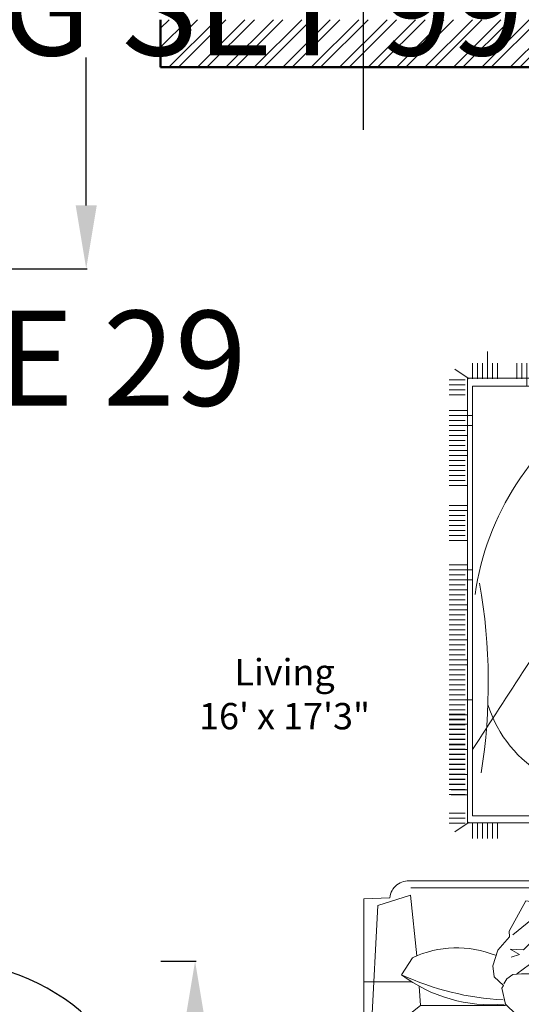
# Model space of a CAD drawing. Units: inches. Extents: x -90 to 536, y -553 to 299.
# Tile 13 of 27: x 206 to 301, y -339 to -153. Entities that reach past the tile are written whole.
import ezdxf

# ---------------------------------------------------------------- set-up
doc = ezdxf.new("R2010")
doc.units = ezdxf.units.IN
for name, color, linetype, lineweight in [('A-ANNO-DIMS', 2, 'Continuous', 18), ('A-AREA-IDEN', 7, 'Continuous', 18), ('A-DOOR', 4, 'Continuous', 25), ('A-WALL-PATT', 252, 'Continuous', 13), ('Furniture', 2, 'Continuous', 18), ('Outer Wall', 1, 'Continuous', 50)]:
    doc.layers.add(name, color=color, linetype=linetype, lineweight=lineweight)
doc.styles.get("Standard").update_dxf_attribs({"font": 'arial.ttf'})
doc.dimstyles.get("Standard").update_dxf_attribs({"dimtxt": 18, "dimasz": 12, "dimexe": 0.18, "dimexo": 0.0625, "dimgap": 0.09, "dimtad": 0, "dimtih": 1, "dimtoh": 1, "dimdec": 0, "dimzin": 0, "dimdsep": 46, "dimlunit": 3, "dimtxsty": 'Standard', "dimcen": 0.09, "dimadec": 0, "dimazin": 0, "dimtfac": 1, "dimtdec": 0, "dimtofl": 0, "dimtmove": 0, "dimatfit": 3, "dimfxl": 1, "dimtolj": 1, "dimtzin": 0, "dimarcsym": 0})

# ---------------------------------------------------------------- blocks, each defined once
blk = doc.blocks.new('A$C4DC51D13')
for p, q in [((3265.3, 2996.2), (1188.4, 2996.2)), ((1188.4, 2962.7), (1862.1, 2962.7)), ((1862.1, 2134), (1862.1, 2962.7)), ((1895.2, 2134), (1895.2, 2996.2)), ((1928.3, 2961.6), (2524.2, 2961.6)), ((1928.3, 2134), (1928.3, 2961.6)), ((2524.2, 2961.6), (2524.2, 2658.6)), ((2559.6, 2996.2), (2559.6, 2617.8)), ((2590.4, 2962.7), (2590.4, 2654.5)), ((3265.3, 2962.7), (2590.4, 2962.7)), ((277.4, 2939.6), (277.4, 2141.8)), ((943, 2103.5), (943, 2936.7)), ((1018.2, 2892.3), (232.2, 2892.3)), ((1290.4, 2664.8), (1028, 2870.9)), ((3163.3, 2664.8), (3425.7, 2870.9)), ((3778.5, 2897), (3631.2, 2747.3)), ((4008.9, 2375.5), (3778.5, 2897)), ((4156.2, 2525.2), (3778.5, 2897)), ((304, 2865.7), (304, 2253.3)), ((916.4, 2865.7), (304, 2865.7)), ((916.4, 2253.3), (916.4, 2865.7)), ((1022.9, 2163.8), (1022.9, 2830.3)), ((1056, 2830.3), (1081, 2194.8)), ((3397.7, 2830.3), (3364.5, 2194.8)), ((3430.8, 2163.8), (3430.8, 2830.3)), ((4008.9, 2375.5), (3631.2, 2747.3)), ((423.7, 2370.8), (776.6, 2723.7)), ((427.4, 2727.4), (772.8, 2367.1)), ((481, 2622.2), (481, 2686.2)), ((485.3, 2628.5), (485.3, 2689.7)), ((489.5, 2634.2), (489.5, 2693)), ((493.7, 2639.3), (493.7, 2696.1)), ((497.9, 2644), (497.9, 2699.1)), ((502.2, 2648.3), (502.2, 2701.8)), ((506.4, 2652.2), (506.4, 2704.4)), ((510.6, 2655.8), (510.6, 2706.9)), ((514.9, 2659.2), (514.9, 2709.2)), ((519.1, 2662.3), (519.1, 2711.3)), ((523.3, 2665.1), (523.3, 2713.4)), ((527.5, 2667.8), (527.5, 2715.2)), ((531.8, 2670.2), (531.8, 2717)), ((536, 2672.5), (536, 2718.7)), ((540.2, 2674.6), (540.2, 2720.2)), ((544.4, 2676.5), (544.4, 2721.6)), ((548.7, 2678.2), (548.7, 2722.9)), ((650.1, 2678.8), (650.1, 2723.3)), ((654.3, 2677.1), (654.3, 2722)), ((658.6, 2675.2), (658.6, 2720.7)), ((662.8, 2673.2), (662.8, 2719.2)), ((667, 2671), (667, 2717.6)), ((668.5, 2670.2), (668.5, 2717)), ((671.2, 2668.6), (671.2, 2715.9)), ((672.7, 2667.8), (672.7, 2715.2)), ((675.5, 2666.1), (675.5, 2714)), ((676.9, 2665.1), (676.9, 2713.4)), ((679.7, 2663.3), (679.7, 2712)), ((681.1, 2662.3), (681.1, 2711.3)), ((683.9, 2660.3), (683.9, 2709.9)), ((685.4, 2659.2), (685.4, 2709.2)), ((688.1, 2657), (688.1, 2707.7)), ((689.6, 2655.8), (689.6, 2706.9)), ((692.4, 2653.5), (692.4, 2705.3)), ((693.8, 2652.2), (693.8, 2704.4)), ((696.6, 2649.6), (696.6, 2702.7)), ((698, 2648.3), (698, 2701.8)), ((700.8, 2645.5), (700.8, 2700)), ((702.3, 2644), (702.3, 2699.1)), ((705, 2641), (705, 2697.2)), ((706.5, 2639.3), (706.5, 2696.1)), ((709.3, 2636), (709.3, 2694.1)), ((710.7, 2634.2), (710.7, 2693)), ((713.5, 2630.5), (713.5, 2690.9)), ((714.9, 2628.5), (714.9, 2689.7)), ((717.7, 2624.4), (717.7, 2687.4)), ((719.2, 2622.2), (719.2, 2686.2)), ((722, 2617.6), (722, 2683.8)), ((441, 2637.7), (492.3, 2637.7)), ((443, 2453.4), (443, 2641.1)), ((443.5, 2641.9), (496, 2641.9)), ((446.1, 2646.1), (500, 2646.1)), ((447.2, 2446.7), (447.2, 2647.8)), ((448.9, 2650.4), (504.4, 2650.4)), ((451.5, 2440.6), (451.5, 2654)), ((451.9, 2654.6), (509.2, 2654.6)), ((455.1, 2658.8), (514.4, 2658.8)), ((455.7, 2434.9), (455.7, 2659.6)), ((458.4, 2663.1), (520.2, 2663.1)), ((459.9, 2558.8), (459.9, 2664.9)), ((462, 2667.3), (526.7, 2667.3)), ((464.1, 2583.3), (464.1, 2669.7)), ((465.8, 2671.5), (534.1, 2671.5)), ((468.4, 2596.6), (468.4, 2674.3)), ((469.8, 2675.7), (542.8, 2675.7)), ((472.6, 2606.7), (472.6, 2678.5)), ((476.8, 2615), (476.8, 2682.5)), ((489.5, 2667.3), (489.5, 2633.5)), ((657.4, 2675.7), (730.4, 2675.7)), ((734.5, 2671.5), (666.1, 2671.5)), ((666.1, 2671.5), (734.5, 2671.5)), ((738.2, 2667.3), (673.5, 2667.3)), ((673.5, 2667.3), (738.2, 2667.3)), ((741.8, 2663.1), (680, 2663.1)), ((680, 2663.1), (741.8, 2663.1)), ((745.2, 2658.8), (685.8, 2658.8)), ((685.8, 2658.8), (745.2, 2658.8)), ((748.3, 2654.6), (691, 2654.6)), ((691, 2654.6), (748.3, 2654.6)), ((751.3, 2650.4), (695.8, 2650.4)), ((695.8, 2650.4), (751.3, 2650.4)), ((754.1, 2646.1), (700.2, 2646.1)), ((700.2, 2646.1), (754.1, 2646.1)), ((756.7, 2641.9), (704.2, 2641.9)), ((704.2, 2641.9), (756.7, 2641.9)), ((759.2, 2637.7), (707.9, 2637.7)), ((707.9, 2637.7), (759.2, 2637.7)), ((723.4, 2615), (723.4, 2682.5)), ((726.2, 2609.7), (726.2, 2679.9)), ((727.6, 2606.7), (727.6, 2678.5)), ((730.4, 2600.3), (730.4, 2675.7)), ((731.9, 2596.6), (731.9, 2674.3)), ((734.6, 2588.4), (734.6, 2671.3)), ((736.1, 2583.3), (736.1, 2669.7)), ((738.9, 2570.4), (738.9, 2666.6)), ((740.3, 2558.8), (740.3, 2664.9)), ((743.1, 2433.1), (743.1, 2661.5)), ((744.5, 2434.9), (744.5, 2659.6)), ((747.3, 2438.6), (747.3, 2656)), ((748.8, 2440.6), (748.8, 2654)), ((751.5, 2444.5), (751.5, 2650)), ((753, 2446.7), (753, 2647.8)), ((755.8, 2451.1), (755.8, 2643.5)), ((757.2, 2453.4), (757.2, 2641.1)), ((1283.3, 2574.2), (1290.4, 2664.8)), ((1290.4, 2664.8), (1894.7, 2664.8)), ((1798, 2530.2), (1812.1, 2637.9)), ((1895.2, 2663.7), (2557.3, 2663.7)), ((2603.6, 2664.8), (2559, 2664.8)), ((3163.3, 2664.8), (2764.7, 2664.8)), ((3170.4, 2574.2), (3163.3, 2664.8)), ((3631.7, 2676.6), (3938.2, 2375)), ((422.5, 2591.2), (466.5, 2591.2)), ((423.6, 2595.4), (467.9, 2595.4)), ((424.8, 2599.7), (469.6, 2599.7)), ((426.1, 2603.9), (471.3, 2603.9)), ((426.1, 2490.7), (426.1, 2603.9)), ((427.5, 2608.1), (473.3, 2608.1)), ((429.1, 2612.3), (475.4, 2612.3)), ((430.3, 2479), (430.3, 2615.5)), ((430.7, 2616.6), (477.7, 2616.6)), ((432.5, 2620.8), (480.2, 2620.8)), ((434.5, 2469.3), (434.5, 2625.2)), ((434.5, 2625), (482.9, 2625)), ((436.5, 2629.2), (485.8, 2629.2)), ((438.7, 2633.5), (488.9, 2633.5)), ((438.8, 2460.9), (438.8, 2633.6)), ((761.5, 2633.5), (711.3, 2633.5)), ((711.3, 2633.5), (761.5, 2633.5)), ((763.7, 2629.2), (714.4, 2629.2)), ((714.4, 2629.2), (763.7, 2629.2)), ((765.8, 2625), (717.3, 2625)), ((767.7, 2620.8), (720, 2620.8)), ((769.5, 2616.6), (722.5, 2616.6)), ((771.1, 2612.3), (724.8, 2612.3)), ((772.7, 2608.1), (726.9, 2608.1)), ((774.1, 2603.9), (728.9, 2603.9)), ((775.4, 2599.7), (730.7, 2599.7)), ((776.6, 2595.4), (732.3, 2595.4)), ((777.7, 2591.2), (733.7, 2591.2)), ((760, 2458.3), (760, 2636.3)), ((761.4, 2460.9), (761.4, 2633.6)), ((764.2, 2466.3), (764.2, 2628.2)), ((765.7, 2469.3), (765.7, 2625.2)), ((417.1, 2548.9), (459.4, 2548.9)), ((417.1, 2544.7), (459.5, 2544.7)), ((417.2, 2553.2), (459.6, 2553.2)), ((417.4, 2557.4), (459.8, 2557.4)), ((417.7, 2561.6), (460.2, 2561.6)), ((418.1, 2565.8), (460.7, 2565.8)), ((418.5, 2570.1), (461.3, 2570.1)), ((419.1, 2574.3), (462.1, 2574.3)), ((419.8, 2578.5), (462.9, 2578.5)), ((420.6, 2582.7), (464, 2582.7)), ((421.5, 2587), (465.2, 2587)), ((778.7, 2587), (735.1, 2587)), ((779.6, 2582.7), (736.2, 2582.7)), ((780.4, 2578.5), (737.3, 2578.5)), ((781.1, 2574.3), (738.2, 2574.3)), ((781.7, 2570.1), (738.9, 2570.1)), ((782.2, 2565.8), (739.6, 2565.8)), ((782.5, 2561.6), (740.1, 2561.6)), ((782.8, 2557.4), (740.4, 2557.4)), ((783, 2553.2), (740.7, 2553.2)), ((783.1, 2548.9), (740.8, 2548.9)), ((783.1, 2544.7), (740.8, 2544.7)), ((1022.9, 2554.4), (1249.6, 2554.4)), ((1895.5, 2582.2), (1932.3, 2494.6)), ((3430.8, 2554.4), (3204.1, 2554.4)), ((417.2, 2540.5), (459.6, 2540.5)), ((417.5, 2536.3), (459.9, 2536.3)), ((417.8, 2532), (460.3, 2532)), ((418.2, 2527.8), (460.8, 2527.8)), ((418.7, 2523.6), (461.4, 2523.6)), ((419.3, 2519.4), (462.2, 2519.4)), ((459.9, 2429.7), (459.9, 2535.7)), ((781, 2519.4), (738, 2519.4)), ((781.6, 2523.6), (738.8, 2523.6)), ((782.1, 2527.8), (739.4, 2527.8)), ((782.5, 2532), (740, 2532)), ((740.3, 2429.7), (740.3, 2535.7)), ((782.8, 2536.3), (740.4, 2536.3)), ((783, 2540.5), (740.6, 2540.5)), ((1200, 2520.5), (1251.9, 2440.8)), ((2559, 2535.8), (2557.3, 2535.8)), ((3253.7, 2520.5), (3201.8, 2440.8)), ((4008.9, 2375.5), (4156.2, 2525.2)), ((1243.2, 2146.7), (1272.2, 2431.8)), ((3210.5, 2146.7), (3181.5, 2431.8)), ((242.9, 2226.7), (1018.2, 2226.7)), ((304, 2253.3), (916.4, 2253.3)), ((1081, 2194.8), (1243.2, 2146.7)), ((3364.5, 2194.8), (3210.5, 2146.7)), ((498.8, 1837.1), (382.1, 2139.5)), ((1040.3, 1942.9), (421.2, 2132.6)), ((1145.1, 2159.3), (1022.9, 2163.8)), ((1145.1, 2159.3), (1243.2, 2146.7)), ((1244.8, 2113), (1243.2, 2146.7)), ((2590.4, 2164.3), (2590.4, 2134)), ((3208.9, 2113), (3210.5, 2146.7)), ((3308.6, 2159.3), (3210.5, 2146.7)), ((3308.6, 2159.3), (3430.8, 2163.8)), ((411.8, 2101.9), (992.6, 1890.2)), ((1839.5, 2113), (1244.8, 2113)), ((2308.5, 2111.9), (1950.4, 2111.9)), ((2614.2, 2113), (3208.9, 2113)), ((677.4, 2054.1), (612.9, 1843.6)), ((1839.5, 2079.9), (1244.8, 2079.9)), ((2322.1, 2078.8), (1950.4, 2078.8)), ((2614.2, 2079.9), (3208.9, 2079.9)), ((220.3, 2026), (19.3, 1370.1)), ((251.1, 2016.6), (37.1, 1314.7)), ((1009.7, 1828.1), (1040.3, 1942.9)), ((658.5, 1880), (717.8, 1809.1)), ((992.6, 1890.2), (993.4, 1733.4)), ((1158.3, 1784.3), (1158.3, 1858.2)), ((1181.8, 1784.3), (1181.8, 1858.2)), ((1205.3, 1784.3), (1205.3, 1858.2)), ((1228.8, 1784.3), (1228.8, 1858.2)), ((1252.2, 1784.3), (1252.2, 1858.2)), ((1319.4, 1784.3), (1319.4, 1858.2)), ((1342.9, 1784.3), (1342.9, 1858.2)), ((1366.3, 1784.3), (1366.3, 1858.2)), ((1389.8, 1784.3), (1389.8, 1858.2)), ((1413.3, 1784.3), (1413.3, 1858.2)), ((1436.8, 1784.3), (1436.8, 1858.2)), ((1460.2, 1784.3), (1460.2, 1858.2)), ((1483.7, 1784.3), (1483.7, 1858.2)), ((1507.2, 1784.3), (1507.2, 1858.2)), ((1530.7, 1784.3), (1530.7, 1858.2)), ((1554.1, 1784.3), (1554.1, 1858.2)), ((1577.6, 1784.3), (1577.6, 1858.2)), ((1714.2, 1784.3), (1714.2, 1858.2)), ((1737.6, 1784.3), (1737.6, 1858.2)), ((1761.1, 1784.3), (1761.1, 1858.2)), ((1784.6, 1784.3), (1784.6, 1858.2)), ((1808.1, 1784.3), (1808.1, 1858.2)), ((1831.5, 1784.3), (1831.5, 1858.2)), ((1855, 1784.3), (1855, 1858.2)), ((1878.5, 1784.3), (1878.5, 1858.2)), ((1902, 1784.3), (1902, 1858.2)), ((2050.7, 1784.3), (2050.7, 1858.2)), ((2074.2, 1784.3), (2074.2, 1858.2)), ((2097.7, 1784.3), (2097.7, 1858.2)), ((2121.1, 1784.3), (2121.1, 1858.2)), ((2144.6, 1784.3), (2144.6, 1858.2)), ((2168.1, 1784.3), (2168.1, 1858.2)), ((2191.6, 1782.4), (2191.6, 1856.3)), ((2238.5, 1785.1), (2238.5, 1859)), ((2262, 1784.3), (2262, 1858.2)), ((2285.4, 1784.3), (2285.4, 1858.2)), ((2543.7, 1784.3), (2543.7, 1858.2)), ((2567.1, 1784.3), (2567.1, 1858.2)), ((2590.6, 1784.3), (2590.6, 1858.2)), ((2614.1, 1784.3), (2614.1, 1858.2)), ((2661, 1784.3), (2661, 1858.2)), ((2684.5, 1784.3), (2684.5, 1858.2)), ((2708, 1772.3), (2708, 1858.2)), ((2731.5, 1784.3), (2731.5, 1858.2)), ((2754.9, 1784.3), (2754.9, 1858.2)), ((2778.4, 1784.3), (2778.4, 1858.2)), ((2801.9, 1784.3), (2801.9, 1858.2)), ((2825.4, 1784.3), (2825.4, 1858.2)), ((2848.8, 1784.3), (2848.8, 1858.2)), ((2872.3, 1784.3), (2872.3, 1858.2)), ((2895.8, 1784.3), (2895.8, 1858.2)), ((2919.3, 1784.3), (2919.3, 1858.2)), ((2942.7, 1784.3), (2942.7, 1858.2)), ((2966.2, 1744.8), (2966.2, 1858.2)), ((2989.7, 1784.3), (2989.7, 1858.2)), ((3013.2, 1772.3), (3013.2, 1858.2)), ((3036.6, 1784.3), (3036.6, 1858.2)), ((3060.1, 1784.3), (3060.1, 1858.2)), ((3083.6, 1784.3), (3083.6, 1858.2)), ((498.8, 1837.1), (341.4, 1323.6)), ((584.9, 1817.9), (498.8, 1837.1)), ((1009.7, 1828.1), (993.4, 1733.4)), ((1158.3, 1821.3), (1158.5, 487.7)), ((2215, 1785.7), (2215, 1832.3)), ((993.4, 1733.4), (720.4, 1787.6)), ((1166.1, 1769.7), (1091.8, 1794.5)), ((3248.4, 1772.3), (1158.5, 1772.3)), ((3248.4, 487.7), (3248.4, 1772.3)), ((3248.8, 1760.8), (3322.7, 1760.8)), ((1024.2, 1722.3), (842.3, 1125.2)), ((873.1, 1115.8), (1055, 1712.9)), ((1024.2, 1722.3), (993.4, 1733.4)), ((1162.1, 1754.9), (1088.2, 1754.9)), ((1162.1, 1741.1), (1088.2, 1741.1)), ((1162.1, 1717.6), (1088.2, 1717.6)), ((1196, 511), (1196, 1744.8)), ((1196, 1744.8), (3215.6, 1744.8)), ((3215.6, 511), (3215.6, 1744.8)), ((3248.8, 1737.3), (3322.7, 1737.3)), ((3248.8, 1713.8), (3322.7, 1713.8)), ((3600.6, 1621.7), (3605.1, 1743.8)), ((3605.1, 1743.8), (4271.6, 1743.8)), ((3995.7, 1743.8), (3995.7, 1517.1)), ((4106.1, 1476.4), (4312.2, 1738.8)), ((1162.1, 1708), (1088.2, 1708)), ((1162.1, 1684.5), (1088.2, 1684.5)), ((3248.8, 1690.4), (3322.7, 1690.4)), ((3248.8, 1666.9), (3322.7, 1666.9)), ((3636.1, 1685.8), (3588, 1523.6)), ((4271.6, 1710.7), (3636.1, 1685.8)), ((3248.8, 1643.4), (3322.7, 1643.4)), ((3248.8, 1619.9), (3322.7, 1619.9)), ((3600.6, 1621.7), (3588, 1523.6)), ((4404, 1578.3), (4404, 904.6)), ((4437.5, 165.9), (4437.5, 1578.3)), ((1701.7, 1530), (1701.7, 911.2)), ((1162.1, 1492.9), (1088.2, 1492.9)), ((1162.1, 1483.3), (1088.2, 1483.3)), ((1737.7, 1483.1), (1737.7, 911.2)), ((2593.1, 907.9), (2593.1, 1490.3)), ((2629.1, 907.9), (2629.1, 1503.1)), ((3248.8, 1513.8), (3322.7, 1513.8)), ((3248.8, 1513.3), (3322.7, 1513.3)), ((3248.8, 1490.4), (3322.7, 1490.4)), ((3248.8, 1489.9), (3322.7, 1489.9)), ((3521.2, 1130.7), (3521.2, 1521.9)), ((3554.3, 1131.4), (3554.3, 1521.9)), ((3588, 1523.6), (3873.1, 1494.5)), ((4015.5, 1483.4), (4106.1, 1476.4)), ((1162.1, 1459.8), (1088.2, 1459.8)), ((1162.1, 1446), (1088.2, 1446)), ((2674.6, 1449.9), (1641, 1449.9)), ((1888.1, 1449.9), (1701.7, 1263.5)), ((1856.2, 1449.9), (1701.7, 1295.4)), ((1715.1, 1449.9), (1701.7, 1436.5)), ((2343.3, 1449.9), (1855.3, 961.9)), ((2629.1, 1449), (2142, 961.9)), ((2325.1, 1449.9), (2154.2, 1279.1)), ((2461.6, 1449.9), (2177, 1165.3)), ((3248.8, 1466.9), (3322.7, 1466.9)), ((3248.8, 1443.4), (3322.7, 1443.4)), ((4106.1, 1476.4), (4106.1, 872.1)), ((1162.1, 1412.8), (1088.2, 1412.8)), ((1162.1, 1399), (1088.2, 1399)), ((2674.6, 1413.9), (1641, 1413.9)), ((3248.8, 1419.9), (3322.7, 1419.9)), ((3250, 1407.8), (3519, 1407.8)), ((6.3, 1324.2), (19.3, 1370.2)), ((479.3, 1327.3), (375.2, 1344.9)), ((1162.1, 1375.5), (1088.2, 1375.5)), ((1162.1, 1352.1), (1088.2, 1352.1)), ((1162.1, 1342.9), (1088.2, 1342.9)), ((1162.1, 1342.4), (1088.2, 1342.4)), ((3248.8, 1359), (3322.7, 1359)), ((342.8, 1324.6), (76.7, 1139.6)), ((843, 1127.6), (342.8, 1324.6)), ((1162.1, 1319.4), (1088.2, 1319.4)), ((1162.1, 1318.9), (1088.2, 1318.9)), ((1162.1, 1296), (1088.2, 1296)), ((1162.1, 1295.5), (1088.2, 1295.5)), ((3248.8, 990.8), (3248.4, 1328.4)), ((3248.8, 1312.1), (3322.7, 1312.1)), ((3248.8, 1302.3), (3322.7, 1302.3)), ((3250, 1317.8), (3519, 1317.8)), ((369.2, 1044.8), (442.9, 1285.2)), ((1196, 1272.5), (1088.2, 1272.5)), ((1162.1, 1272), (1088.2, 1272)), ((2629.1, 1280.5), (2310.5, 961.9)), ((1162.1, 1249), (1088.2, 1249)), ((1162.1, 1248.5), (1088.2, 1248.5)), ((1162.1, 1225.5), (1088.2, 1225.5)), ((3248.8, 1249), (3322.7, 1249)), ((3248.8, 1248.5), (3322.7, 1248.5)), ((3248.8, 1239.3), (3322.7, 1239.3)), ((3248.8, 1238.8), (3322.7, 1238.8)), ((3248.8, 1225.5), (3322.7, 1225.5)), ((1162.1, 1202.1), (1088.2, 1202.1)), ((1196, 1178.6), (1088.2, 1178.6)), ((1728.6, 1158.4), (1701.7, 1131.5)), ((3248.8, 1202.1), (3322.7, 1202.1)), ((3248.8, 1178.6), (3322.7, 1178.6)), ((732, 933.5), (112.9, 1123.3)), ((122.4, 1154.1), (719.7, 996.3)), ((719.7, 996.3), (810.6, 1133.2)), ((771, 1045.7), (810.6, 1133.2)), ((842.3, 1125.2), (810.6, 1133.2)), ((1162.1, 1155.1), (1088.2, 1155.1)), ((1162.1, 1131.6), (1088.2, 1131.6)), ((3248.8, 1155.1), (3322.7, 1155.1)), ((3248.8, 1131.6), (3322.7, 1131.6)), ((1162.1, 1108.2), (1088.2, 1108.2)), ((1162.1, 1084.7), (1088.2, 1084.7)), ((3248.8, 1108.2), (3322.7, 1108.2)), ((771, 1045.7), (732, 933.5)), ((1196, 1061.2), (1088.2, 1061.2)), ((1162.1, 1037.7), (1088.2, 1037.7)), ((1648.3, 1019.6), (2616.7, 1019.6)), ((1926.6, 1051.5), (1837.1, 961.9)), ((1162.1, 1014.3), (1088.2, 1014.3)), ((2006.3, 994.6), (1973.6, 961.9)), ((2459.2, 974.1), (2447, 961.9)), ((2629.1, 1012), (2579, 961.9)), ((3248.8, 1014.3), (3322.7, 1014.3)), ((3248.8, 990.8), (3322.7, 990.8)), ((1196, 967.3), (1088.2, 967.3)), ((1162.1, 943.8), (1088.2, 943.8)), ((1648.3, 961.9), (2681.9, 961.9)), ((3248.8, 967.3), (3322.7, 967.3)), ((3248.8, 943.8), (3322.7, 943.8)), ((1162.1, 920.4), (1088.2, 920.4)), ((3248.8, 920.4), (3322.7, 920.4)), ((4097.4, 904.6), (4404, 904.6)), ((1196, 860.5), (1088.2, 860.5)), ((1162.1, 837), (1088.2, 837)), ((4106.1, 871.5), (4437.5, 871.5)), ((4404, 840.7), (4110.5, 840.7)), ((4404, 165.9), (4404, 840.7)), ((1162.1, 790), (1031.8, 790)), ((1162.1, 813.5), (1088.2, 813.5)), ((3521.2, 816.9), (3521.2, 222.3)), ((3554.3, 816.9), (3554.3, 222.3)), ((1196, 766.6), (1088.2, 766.6)), ((1162.1, 743.1), (1088.2, 743.1)), ((1162.1, 719.6), (1088.2, 719.6)), ((4106.1, 267.8), (4106.1, 666.5)), ((1162.1, 627.8), (1088.2, 627.8)), ((1162.1, 604.4), (1088.2, 604.4)), ((3248.8, 627.8), (3322.7, 627.8)), ((3248.8, 604.4), (3322.7, 604.4)), ((1162.1, 580.9), (1034.2, 580.9)), ((1162.1, 557.4), (1088.2, 557.4)), ((3248.8, 580.9), (3322.7, 580.9)), ((3248.8, 557.4), (3322.7, 557.4)), ((1162.1, 533.9), (1088.2, 533.9)), ((1162.1, 510.5), (1088.2, 510.5)), ((3215.6, 511), (1196, 511)), ((1334.6, 511), (1334.6, 402.4)), ((1381.6, 511), (1381.6, 402.4)), ((2059.5, 511), (2059.5, 402.4)), ((2106.4, 511), (2106.4, 402.4)), ((2669.8, 511), (2669.8, 402.4)), ((3248.8, 533.9), (3322.7, 533.9)), ((3248.8, 510.5), (3322.7, 510.5)), ((1162, 495.1), (1116.6, 429)), ((1158.5, 487.7), (3248.4, 487.7)), ((1167.1, 476.3), (1167.1, 402.4)), ((1190.6, 476.3), (1190.6, 402.4)), ((1214, 476.3), (1214, 402.4)), ((1237.5, 476.3), (1237.5, 402.4)), ((1311.1, 487.7), (1311.1, 402.4)), ((1358.1, 476.3), (1358.1, 402.4)), ((1405, 476.3), (1405, 402.4)), ((1428.5, 487.7), (1428.5, 402.4)), ((1452, 476.3), (1452, 402.4)), ((1475.5, 476.3), (1475.5, 402.4)), ((1498.9, 487.7), (1498.9, 402.4)), ((1522.4, 487.7), (1522.4, 402.4)), ((1545.9, 476.3), (1545.9, 402.4)), ((1569.4, 476.3), (1569.4, 402.4)), ((1592.8, 476.3), (1592.8, 402.4)), ((1616.3, 476.3), (1616.3, 402.4)), ((1639.8, 476.3), (1639.8, 402.4)), ((1663.3, 487.7), (1663.3, 402.4)), ((1757.8, 487.7), (1757.8, 402.4)), ((1781.3, 487.7), (1781.3, 402.4)), ((1804.8, 476.3), (1804.8, 402.4)), ((1828.2, 476.3), (1828.2, 402.4)), ((1851.7, 476.3), (1851.7, 402.4)), ((1875.2, 476.3), (1875.2, 402.4)), ((1898.7, 476.3), (1898.7, 402.4)), ((1922.1, 487.7), (1922.1, 402.4)), ((2036, 487.7), (2036, 402.4)), ((2082.9, 476.3), (2082.9, 402.4)), ((2129.9, 476.3), (2129.9, 402.4)), ((2153.4, 487.7), (2153.4, 402.4)), ((2176.8, 476.3), (2176.8, 402.4)), ((2200.3, 476.3), (2200.3, 402.4)), ((2223.8, 487.7), (2223.8, 402.4)), ((2247.2, 487.7), (2247.2, 402.4)), ((2270.7, 476.3), (2270.7, 402.4)), ((2294.2, 476.3), (2294.2, 402.4)), ((2317.7, 476.3), (2317.7, 402.4)), ((2341.1, 476.3), (2341.1, 402.4)), ((2364.6, 476.3), (2364.6, 402.4)), ((2388.1, 487.7), (2388.1, 402.4)), ((2411.6, 476.3), (2411.6, 402.4)), ((2435, 476.3), (2435, 402.4)), ((2458.5, 476.3), (2458.5, 402.4)), ((2482, 487.7), (2482, 402.4)), ((2505.5, 487.7), (2505.5, 402.4)), ((2528.9, 476.3), (2528.9, 402.4)), ((2552.4, 476.3), (2552.4, 402.4)), ((2575.9, 476.3), (2575.9, 402.4)), ((2599.4, 476.3), (2599.4, 402.4)), ((2622.8, 476.3), (2622.8, 402.4)), ((2646.3, 476.3), (2646.3, 402.4)), ((2693.3, 476.3), (2693.3, 402.4)), ((2716.7, 476.3), (2716.7, 402.4)), ((2738, 476.3), (2738, 402.4)), ((2740.2, 487.7), (2740.2, 402.4)), ((2761.5, 476.3), (2761.5, 402.4)), ((2763.7, 476.3), (2763.7, 402.4)), ((2784.9, 487.7), (2784.9, 402.4)), ((2787.2, 476.3), (2787.2, 402.4)), ((2808.4, 476.3), (2808.4, 402.4)), ((2810.6, 476.3), (2810.6, 402.4)), ((2831.9, 476.3), (2831.9, 402.4)), ((2834.1, 476.3), (2834.1, 402.4)), ((2855.4, 476.3), (2855.4, 402.4)), ((2857.6, 476.3), (2857.6, 402.4)), ((2878.8, 476.3), (2878.8, 402.4)), ((2881.1, 476.3), (2881.1, 402.4)), ((2902.3, 476.3), (2902.3, 402.4)), ((2904.5, 487.7), (2904.5, 402.4)), ((2925.8, 476.3), (2925.8, 402.4)), ((2928, 476.3), (2928, 402.4)), ((2949.3, 476.3), (2949.3, 402.4)), ((2951.5, 476.3), (2951.5, 402.4)), ((2972.7, 476.3), (2972.7, 402.4)), ((2975, 476.3), (2975, 402.4)), ((2996.2, 476.3), (2996.2, 402.4)), ((2998.4, 476.3), (2998.4, 402.4)), ((3019.7, 476.3), (3019.7, 402.4)), ((3021.9, 487.7), (3021.9, 402.4)), ((3043.2, 476.3), (3043.2, 402.4)), ((3045.4, 476.3), (3045.4, 402.4)), ((3066.6, 476.3), (3066.6, 402.4)), ((3068.9, 476.3), (3068.9, 402.4)), ((3092.3, 476.3), (3092.3, 402.4)), ((3092.7, 484.5), (3092.7, 410.6)), ((3115.8, 476.3), (3115.8, 402.4)), ((3116.2, 484.5), (3116.2, 410.6)), ((3202.2, 476.3), (3202.2, 402.4)), ((3225.7, 476.3), (3225.7, 402.4)), ((3244.9, 495.1), (3290.3, 429)), ((3249.2, 476.3), (3249.2, 402.4)), ((3588, 220.6), (3873.1, 249.7)), ((4015.5, 260.8), (4106.1, 267.8)), ((4106.1, 267.8), (4312.2, 5.4)), ((3636.1, 66.6), (3588, 220.6)), ((3961.8, 177.4), (3882.1, 229.3)), ((3995.7, 0.4), (3995.7, 227)), ((3600.6, 122.5), (3605.1, 0.4)), ((4271.6, 33.5), (3636.1, 66.6)), ((3605.1, 0.4), (4271.6, 0.4))]:
    blk.add_line(p, q)
at = {"linetype": 'ByBlock'}
for points in [[(2342.9, 1843.9), (2352.5, 1810.4), (2340.1, 1777.7), (2351.8, 1757), (2412.3, 1818), (2433.1, 1866.4), (2453.1, 1889.5), (2436, 1914.7), (2407.6, 1926.2), (2433.7, 1959.9), (2473.1, 2048.3), (2530.6, 2101.1), (2625.9, 2180.3), (2669, 2174.2), (2748.1, 2315.4), (2745.8, 2342.6), (2801.2, 2404.9), (2823.9, 2479.6), (2818.4, 2529.9), (2775.1, 2571.7), (2782.4, 2583.3), (2765.2, 2658.8), (2714.5, 2706.9), (2634.6, 2708.6), (2571.9, 2652.6), (2548.8, 2649.4), (2474, 2672.1), (2312.9, 2542.1), (2312.9, 2341.6), (2333.9, 2336.4), (2302, 2223.9), (2313.6, 2216.6), (2297.4, 2095.7), (2309.3, 2034.9), (2320.2, 1952), (2319.3, 1929.9), (2280.8, 1863.6), (2257.7, 1842.4), (2239.2, 1825.7), (2220.1, 1798.2), (2221.6, 1713.1), (2254.3, 1700.7), (2275.9, 1729.8), (2288.6, 1768), (2313.7, 1797.6)], [(3285.2, 1088.3), (3251.7, 1078.6), (3219, 1091.1), (3198.3, 1079.4), (3259.3, 1018.8), (3307.7, 998), (3330.8, 978), (3356, 995.1), (3367.5, 1023.6), (3401.2, 997.5), (3489.6, 958), (3542.4, 900.5), (3621.6, 805.3), (3615.5, 762.2), (3756.7, 683), (3783.9, 685.3), (3846.2, 629.9), (3920.9, 607.2), (3971.2, 612.7), (4013, 656), (4024.6, 648.7), (4100.1, 665.9), (4148.2, 716.6), (4149.9, 796.5), (4093.9, 859.3), (4090.7, 882.4), (4113.4, 957.1), (3983.4, 1118.2), (3782.9, 1118.2), (3777.7, 1097.2), (3665.2, 1129.2), (3657.9, 1117.6), (3537, 1133.7), (3476.2, 1121.9), (3393.3, 1110.9), (3371.2, 1111.9), (3304.9, 1150.4), (3283.7, 1173.4), (3267, 1191.9), (3239.5, 1211), (3154.4, 1209.5), (3142, 1176.8), (3171.1, 1155.3), (3209.3, 1142.5), (3238.9, 1117.5)]]:
    blk.add_lwpolyline(points, close=True, dxfattribs=at)
for points in [[(2563.4, 2654.7), (2512.2, 2609.3), (2506.2, 2548.3), (2540.1, 2504.4), (2576.9, 2490.9), (2579.8, 2539.3), (2598.7, 2543.6), (2636.7, 2516.4), (2690.3, 2516.7), (2731.2, 2520.1), (2758.5, 2540.1), (2773, 2563.3)], [(2629.1, 2357.8), (2507, 2405.5), (2433.2, 2450.3), (2445.5, 2500.8), (2478.9, 2546.1), (2402.4, 2506.9), (2373.4, 2424.8), (2384.4, 2341.9), (2352.8, 2340.7)], [(2712.3, 2515.8), (2652.7, 2472.4), (2603.2, 2489), (2580, 2503.6)], [(2738, 2438.2), (2699.2, 2425.4), (2742.4, 2401.4), (2680.4, 2403.2), (2604.1, 2328.3), (2519.2, 2273.3), (2529.8, 2261.8), (2402.7, 2252.7), (2395.4, 2241.1), (2431.1, 2241.3), (2375.7, 2196.9), (2385.2, 2181.2), (2474.4, 2199.5), (2549.9, 2234.6), (2596.2, 2223.2), (2730.1, 2333.1)], [(2433.2, 2450.3), (2377.6, 2423.8)], [(2409.5, 2153), (2387.5, 2153.9), (2359, 2165.4), (2352.6, 2193.7), (2353.5, 2215.7), (2330.5, 2194.6), (2322.1, 2196.7), (2341.8, 2240.9), (2345.5, 2329.1)], [(2374.9, 2339.8), (2395.2, 2276.9)], [(2431.4, 2187.8), (2379.5, 2066.7), (2320.2, 1929.7)], [(2613.2, 2183.4), (2541.6, 2218.8)], [(2407.6, 1926.2), (2342.9, 1843.9)], [(2412.9, 1911.5), (2401.6, 1865.2), (2361.9, 1812.5)], [(2279.2, 1765.9), (2259.2, 1757.4), (2247.6, 1764.7), (2246.4, 1796.2), (2253.5, 1843.5)], [(3207.2, 1152), (3198.7, 1171.9), (3206, 1183.5), (3237.5, 1184.7), (3284.8, 1177.6)], [(3629.1, 999.7), (3508, 1051.6), (3371, 1110.9)], [(3352.8, 1018.2), (3306.5, 1029.5), (3253.8, 1069.2)], [(3367.5, 1023.6), (3285.2, 1088.3)], [(3594.3, 1021.6), (3595.2, 1043.7), (3606.7, 1072.1), (3635, 1078.6), (3657, 1077.6), (3635.9, 1100.6), (3638, 1109.1), (3682.2, 1089.3), (3770.4, 1085.6)], [(3799.1, 802), (3846.8, 924.2), (3891.6, 998), (3942.1, 985.6), (3987.4, 952.2), (3948.2, 1028.7), (3866.1, 1057.7), (3783.2, 1046.8), (3782, 1078.3)], [(3879.5, 693.2), (3866.7, 732), (3842.7, 688.8), (3844.5, 750.8), (3769.6, 827.1), (3714.6, 911.9), (3703.1, 901.3), (3694, 1028.4), (3682.4, 1035.7), (3682.6, 1000), (3638.2, 1055.5), (3622.5, 1045.9), (3640.8, 956.7), (3675.9, 881.2), (3664.5, 834.9), (3774.4, 701)], [(3781.1, 1056.2), (3718.2, 1035.9)], [(3891.6, 998), (3865.1, 1053.5)], [(3624.7, 817.9), (3660.1, 889.6)], [(4096, 867.7), (4050.6, 918.9), (3989.6, 924.9), (3945.7, 891.1), (3932.2, 854.2), (3980.6, 851.3), (3984.9, 832.4), (3957.7, 794.4), (3958, 740.9), (3961.4, 699.9), (3981.4, 672.7), (4004.6, 658.1)], [(3957.1, 718.8), (3913.7, 778.5), (3930.3, 827.9), (3944.9, 851.1)]]:
    blk.add_lwpolyline(points, dxfattribs=at)
for centre, radius in [((600.1, 2547.3), 183), ((600.1, 2547.3), 140.7), ((1803.2, 1372.6), 25.7), ((2527.6, 1372.6), 25.7), ((1803.2, 1039.3), 25.7), ((2527.6, 1039.3), 25.7), ((2817.9, 923.4), 31.7), ((2095.7, 858), 41)]:
    blk.add_circle(centre, radius)
for centre, radius, start, end in [((1188.4, 2830.3), 165.9, 90, 180), ((1188.4, 2830.3), 132.4, 90, 180), ((3265.3, 2830.3), 165.9, 0, 90), ((3265.3, 2830.3), 132.4, 0, 90), ((3666.8, 2712.2), 50, 135.4503, 225.4503), ((1626.8, 1949.8), 712.7, 74.928, 126.7929), ((1707.9, 1527), 1115.8, 84.6406, 117.0804), ((2192.2, 2032.6), 624.6, 69.4145, 118.3621), ((2633.9, 373.6), 2292.5, 91.8726, 91.9144), ((2832.8, 1963.1), 698.5, 52.9389, 95.0789), ((2713.3, 1357.7), 1282.3, 65.0725, 87.2152), ((2210.2, 1780.8), 852.5, 76.866, 111.6839), ((1459.9, 2882.7), 488.4, 244.7866, 313.8058), ((2216, 2892.1), 488.4, 234.4888, 282.1285), ((2993.8, 2882.7), 488.4, 248.2152, 295.2134), ((3973.2, 2410.6), 50, 225.4503, 315.4503), ((374.1, 1978.9), 160.8, 72.9571, 162.9571), ((1234.5, 2169.3), 90, 186.4251, 276.5821), ((1839.5, 2135.1), 22.1, 270, 0), ((1839.5, 2135.1), 55.2, 270, 0), ((1950.4, 2134), 55.2, 180, 270), ((1950.4, 2134), 22.1, 180, 270), ((2619.6, 2148.3), 68.5, 191.0595, 265.4426), ((2614.2, 2135.1), 22.1, 180, 270), ((3219.2, 2169.3), 90, 263.4179, 353.5749), ((374.1, 1978.9), 128.6, 72.9571, 162.9571), ((1584.7, 1047), 1245.7, 138.0296, 166.1636), ((1067.1, 1321), 692.3, 126.1642, 178.0291), ((248.2, 1741.7), 474.4, 299.1514, 8.1705), ((974.8, 1747.9), 87.4, 336.375, 66.532), ((4271.6, 1578.3), 165.9, 0, 90), ((4271.6, 1578.3), 132.4, 0, 90), ((944.2, 1233.8), 467.1, 309.4804, 56.621), ((3610.6, 1532.2), 90, 96.4251, 186.5821), ((3383, 1136.2), 721.4, 348.1046, 36.6442), ((2968.3, 1058.8), 1115.8, 356.7543, 27.0804), ((4324, 1306.8), 488.4, 154.7866, 202.7137), ((160.1, 1277), 160.8, 162.9571, 252.9571), ((160.1, 1277), 128.6, 162.9571, 252.9571), ((2517.5, 1143.6), 586.7, 287.3395, 13.1463), ((787.1, 1131.7), 87.4, 259.3822, 349.5393), ((2356.9, 1798.1), 1287.8, 212.1153, 261.9323), ((-29968.2, -49615.7), 59944, 56.743614, 57.623407), ((3404.4, 598.4), 698.5, 322.9389, 5.0789), ((2799, 717.9), 1282.3, 335.0725, 357.2152), ((4324, 437.4), 488.4, 158.2152, 205.2134), ((2591.9, -2109.1), 2694.5, 80.9842, 100.0261), ((3610.6, 212), 90, 173.4179, 263.5749), ((4271.6, 165.9), 132.4, 270, 0), ((4271.6, 165.9), 165.9, 270, 0)]:
    blk.add_arc(centre, radius, start, end)
blk = doc.blocks.new('DOOR-42')
for points in [[(0.75, 3), (0.75, 43.5), (1.5, 43.5), (1.5, 3)], [(0, 0), (1.5, 0), (1.5, 1.5), (0.75, 1.5), (0.75, 3), (0, 3)], [(42, 0), (40.5, 0), (40.5, 1.5), (41.25, 1.5), (41.25, 3), (42, 3)]]:
    blk.add_lwpolyline(points, close=True)
blk.add_arc((0.74, 3), 40.51, 0, 88.9291)
blk = doc.blocks.new('*D35')
at = {"layer": 'A-ANNO-DIMS', "color": 0, "lineweight": -2, "transparency": 16777216}
for p, q in [((233.19, -331.05), (239.84, -331.05)), ((239.66, -343.05), (239.66, -343.4)), ((239.66, -362.55), (239.66, -362.21)), ((233.19, -374.55), (239.84, -374.55))]:
    blk.add_line(p, q, dxfattribs=at)
at = {"layer": 'A-ANNO-DIMS', "color": 0, "transparency": 16777216}
for points in [[(237.66, -343.05), (241.66, -343.05), (239.66, -331.05)], [(237.66, -362.55), (241.66, -362.55), (239.66, -374.55)]]:
    blk.add_solid(points, dxfattribs=at)
at = {"layer": 'Defpoints', "color": 0, "transparency": 16777216}
for p in [(233.13, -331.05), (239.66, -331.05), (233.13, -374.55)]:
    blk.add_point(p, dxfattribs=at)
at = {"layer": 'A-ANNO-DIMS', "color": 0, "transparency": 16777216, "insert": (239.66, -352.8), "char_height": 18, "attachment_point": 5}
blk.add_mtext('\\A1;ENTRY DOOR 44 TYP.', dxfattribs=at)
blk = doc.blocks.new('*D41')
at = {"layer": 'A-ANNO-DIMS', "color": 0, "lineweight": -2, "transparency": 16777216}
for p, q in [((204.27, -100.92), (219.21, -100.92)), ((219.03, -112.92), (219.03, -140.95)), ((219.03, -187.77), (219.03, -159.74)), ((204.27, -199.77), (219.21, -199.77))]:
    blk.add_line(p, q, dxfattribs=at)
at = {"layer": 'A-ANNO-DIMS', "color": 0, "transparency": 16777216}
for points in [[(217.03, -112.92), (221.03, -112.92), (219.03, -100.92)], [(217.03, -187.77), (221.03, -187.77), (219.03, -199.77)]]:
    blk.add_solid(points, dxfattribs=at)
at = {"layer": 'Defpoints', "color": 0, "transparency": 16777216}
for p in [(204.21, -100.92), (219.03, -100.92), (204.21, -199.77)]:
    blk.add_point(p, dxfattribs=at)
at = {"layer": 'A-ANNO-DIMS', "color": 0, "transparency": 16777216, "insert": (219.03, -150.34), "char_height": 18, "attachment_point": 5}
blk.add_mtext('\\A1;DINING SET 99', dxfattribs=at)
blk = doc.blocks.new('*D44')
at = {"layer": 'A-ANNO-DIMS', "color": 0, "lineweight": -2, "transparency": 16777216}
for p, q in [((271.59, -173.44), (271.59, -146.42)), ((283.59, -146.6), (314.65, -146.6)), ((380.5, -146.6), (349.43, -146.6)), ((392.5, -173.44), (392.5, -146.42))]:
    blk.add_line(p, q, dxfattribs=at)
at = {"layer": 'A-ANNO-DIMS', "color": 0, "transparency": 16777216}
for points in [[(283.59, -144.6), (283.59, -148.6), (271.59, -146.6)], [(380.5, -144.6), (380.5, -148.6), (392.5, -146.6)]]:
    blk.add_solid(points, dxfattribs=at)
at = {"layer": 'Defpoints', "color": 0, "transparency": 16777216}
for p in [(392.5, -146.6), (271.59, -173.5), (392.5, -173.5)]:
    blk.add_point(p, dxfattribs=at)
at = {"layer": 'A-ANNO-DIMS', "color": 0, "transparency": 16777216, "insert": (332.04, -146.6), "char_height": 18, "attachment_point": 5}
blk.add_mtext('\\A1;121', dxfattribs=at)
blk = doc.blocks.new('*D49')
at = {"layer": 'A-ANNO-DIMS', "color": 0, "lineweight": -2, "transparency": 16777216}
for p, q in [((115.28, -228.74), (115.28, -216.74)), ((115.28, -216.74), (127.28, -216.74)), ((111.06, -228.74), (115.46, -228.74)), ((115.28, -245.31), (115.28, -240.74)), ((111.06, -257.31), (115.46, -257.31))]:
    blk.add_line(p, q, dxfattribs=at)
at = {"layer": 'A-ANNO-DIMS', "color": 0, "transparency": 16777216}
for points in [[(113.28, -240.74), (117.28, -240.74), (115.28, -228.74)], [(113.28, -245.31), (117.28, -245.31), (115.28, -257.31)]]:
    blk.add_solid(points, dxfattribs=at)
at = {"layer": 'Defpoints', "color": 0, "transparency": 16777216}
for p in [(111, -228.74), (115.28, -228.74), (111, -257.31)]:
    blk.add_point(p, dxfattribs=at)
at = {"layer": 'A-ANNO-DIMS', "color": 0, "transparency": 16777216, "insert": (190.77, -216.74), "char_height": 18, "attachment_point": 5}
blk.add_mtext('\\A1;FRIDGE 29', dxfattribs=at)

msp = doc.modelspace()

# ---------------------------------------------------------------- hatches: boundary and pattern name
at = {"layer": 'A-WALL-PATT'}
h = msp.add_hatch(dxfattribs=at)
h.set_pattern_fill('ANSI32', color=256, scale=0.4)
h.set_pattern_definition([(45, (-88.8105, -603.6155), (-2.694077, 2.694077), []), (45, (-87.0145, -603.6155), (-2.694077, 2.694077), [])])
h.paths.add_polyline_path([(285.1317, 246.4462), (131.1317, 246.4462), (131.1317, 237.4462), (285.1317, 237.4462)])
h.paths.add_polyline_path([(122.1317, 237.4462), (113.1317, 237.4462), (113.1317, 152.4462), (122.1317, 152.4462), (122.1317, 166.4704)])
h.paths.add_polyline_path([(303.1317, 237.4462), (294.1317, 237.4462), (294.1317, 152.4462), (303.1317, 152.4462)])
h.paths.add_polyline_path([(47.1317, 91.9277), (38.1317, 91.9277), (38.1317, -6.5538), (77.1317, -6.5538), (77.1317, 2.4462), (70.5655, 2.4462), (47.1317, 2.4462)])
h.paths.add_polyline_path([(83.052, -61.5538), (47.1317, -61.5538), (47.1317, -24.5538), (38.1317, -24.5538), (38.1317, -70.5538), (74.052, -70.5538), (74.052, -223.5538), (38.1317, -223.5538), (38.1317, -503.5538), (92.1317, -503.5538), (92.1317, -437.5538), (191.1317, -437.5538), (191.1317, -428.5538), (83.1317, -428.5538), (83.1317, -494.5538), (47.1317, -494.5538), (47.1317, -232.5538), (83.052, -232.5538), (83.052, -70.5538)])
h.paths.add_polyline_path([(407.1317, -63.5538), (381.1317, -63.5538), (381.1317, 91.9277), (372.1317, 91.9277), (372.1317, 32.8805), (372.1317, -63.5538), (306.5745, -63.5538), (237.1317, -63.5538), (237.1317, -38.5538), (233.1317, -38.5538), (233.1317, -71.5538), (398.1317, -71.5538), (398.1317, -152.5538), (233.1317, -152.5538), (233.1317, -161.5538), (398.1317, -161.5538), (398.1317, -368.5538), (233.1317, -368.5538), (233.1317, -377.5538), (407.1317, -377.5538), (407.1317, -161.5538)])
h.paths.add_polyline_path([(261.1317, -422.5538), (252.1317, -422.5538), (252.1317, -428.5538), (233.1317, -428.5538), (233.1317, -437.5538), (261.1317, -437.5538)])
h.paths.add_polyline_path([(191.1317, -368.5538), (180.1317, -368.5538), (180.1317, -335.5538), (131.5919, -335.5538), (131.5919, -344.5538), (171.1317, -344.5538), (171.1317, -392.5538), (180.1317, -392.5538), (180.1317, -377.5538), (191.1317, -377.5538)], flags=17)
h.paths.add_polyline_path([(180.1317, -223.5538), (152.1317, -223.5538), (152.1317, -227.5538), (176.1317, -227.5538), (176.1317, -335.5538), (180.1317, -335.5538)], flags=17)
h.paths.add_polyline_path([(131.5919, -335.5538), (83.1317, -335.5538), (83.1317, -339.5538), (83.1317, -392.5538), (87.1317, -392.5538), (87.1317, -339.5538), (131.5919, -339.5538)], flags=17)
h.paths.add_polyline_path([(197.1317, 2.4462), (77.1317, 2.4462), (77.1317, -1.5538), (113.1317, -1.5538), (113.1317, -71.5538), (181.1317, -71.5538), (181.1317, -67.5538), (117.1317, -67.5538), (117.1317, -1.5538), (177.1317, -1.5538), (177.1317, -37.5538), (181.1317, -37.5538), (181.1317, -1.5538), (197.1317, -1.5538)])
h.paths.add_polyline_path([(173.1317, 138.4462), (122.1317, 138.4462), (122.1317, 134.4462), (173.1317, 134.4462)])
h.paths.add_polyline_path([(213.1317, 237.4462), (209.1317, 237.4462), (209.1317, 134.4462), (233.1317, 134.4462), (233.1317, 68.8889), (233.1317, -2.5538), (237.1317, -2.5538), (237.1317, 134.4462), (258.1317, 134.4462), (258.1317, 138.4462), (213.1317, 138.4462)])

# ---------------------------------------------------------------- linework, layer by layer
at = {"layer": 'Outer Wall'}
for p, q in [((233.1317, -161.5538), (233.1317, -152.5538)), ((398.1317, -161.5538), (233.1317, -161.5538))]:
    msp.add_line(p, q, dxfattribs=at)

# ---------------------------------------------------------------- block references
at = {"layer": 'A-DOOR'}
msp.add_blockref('DOOR-42', (191.1317, -374.5538), dxfattribs=at)
at = {"layer": 'Furniture', "xscale": 0.0403522857994069, "yscale": 0.0403522857994069, "zscale": 0.0403522857994069, "rotation": 270}
msp.add_blockref('A$C4DC51D13', (271.5922, -173.7477), dxfattribs=at)

# ---------------------------------------------------------------- texts
at = {"layer": 'A-AREA-IDEN', "insert": (281.2799, -273.7659), "char_height": 5, "attachment_point": 3}
msp.add_mtext_dynamic_manual_height_columns('\\pxqc;{\\fTimes New Roman|b0|i0|c0|p18;Living\\P16\' x 17\'3"}', width=49.342153, gutter_width=12.5, heights=[0], dxfattribs=at)

# ---------------------------------------------------------------- dimensions: what is measured, and where the dimension line sits
at = {"layer": 'A-ANNO-DIMS'}
for base, p1, p2, text, picture, middle in [((219.0345, -100.9205), (204.2077, -199.766), (204.2077, -100.9205), 'DINING SET <>', '*D41', (219.0345, -150.3432)), ((115.2843, -228.7447), (110.9988, -257.3147), (110.9988, -228.7447), 'FRIDGE <>', '*D49', (190.7672, -216.7447)), ((239.6567404714, -331.0537825705), (233.1317404714, -374.5537825705), (233.1317404714, -331.0537825705), 'ENTRY DOOR <> TYP.', '*D35', (239.6567404714, -352.8037825705))]:
    dim = msp.add_linear_dim(base=base, p1=p1, p2=p2, angle=90, text=text, dimstyle='Standard', override={"dimdec": 0, "dimlfac": 1, "dimrnd": 0, "dimzin": 0, "dimdsep": 46, "dimlunit": 2}, dxfattribs=at)
    dim.commit()
    dim.dimension.update_dxf_attribs({"geometry": picture, "text_midpoint": middle})
dim = msp.add_linear_dim(base=(392.4952, -146.6021), p1=(271.5922, -173.4988), p2=(392.4952, -173.4988), dimstyle='Standard', override={"dimdec": 0, "dimlfac": 1, "dimrnd": 0, "dimzin": 0, "dimdsep": 46, "dimlunit": 2}, dxfattribs=at)
dim.commit()
dim.dimension.update_dxf_attribs({"geometry": '*D44', "text_midpoint": (332.0437, -146.6021)})

doc.saveas('drawing.dxf')
